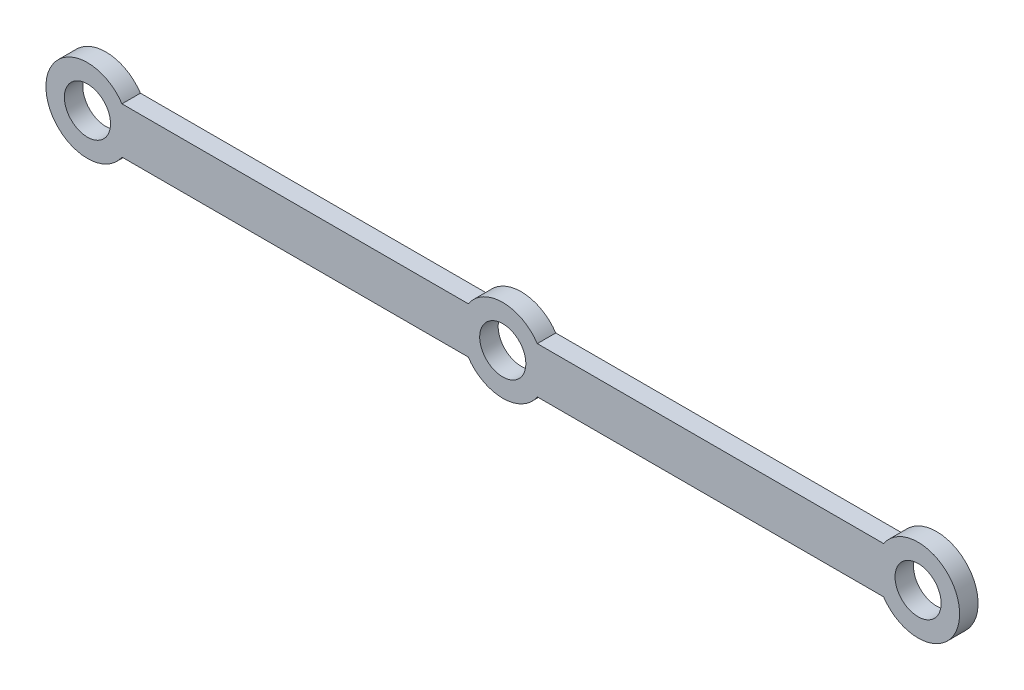
from build123d import *

# Parameters (mm, degrees)
LINK_PROFILE_SKETCH_R = 2.5
LINK_PLATE_2MM_DEPTH  = 1


with BuildPart() as part:
    # Link Profile Sketch → Link Plate 2mm (new, symmetric)
    with BuildSketch(Plane.XY):
        with BuildLine():
            Line((3.741657387, 2.5), (41.258342613, 2.5))
            ThreePointArc((41.258342613, 2.5), (49.5, 0), (41.258342613, -2.5))
            Line((41.258342613, -2.5), (3.741657387, -2.5))
            ThreePointArc((3.741657387, -2.5), (0, -4.5), (-3.741657387, -2.5))
            Line((-3.741657387, -2.5), (-41.258342613, -2.5))
            ThreePointArc((-41.258342613, -2.5), (-49.5, 0), (-41.258342613, 2.5))
            Line((-41.258342613, 2.5), (-3.741657387, 2.5))
            ThreePointArc((-3.741657387, 2.5), (0, 4.5), (3.741657387, 2.5))
        make_face()
        with Locations((-45, 0)):
            Circle(LINK_PROFILE_SKETCH_R, mode=Mode.SUBTRACT)
        Circle(LINK_PROFILE_SKETCH_R, mode=Mode.SUBTRACT)
        with Locations((45, 0)):
            Circle(LINK_PROFILE_SKETCH_R, mode=Mode.SUBTRACT)
    extrude(amount=LINK_PLATE_2MM_DEPTH, both=True)


solid = part.part
